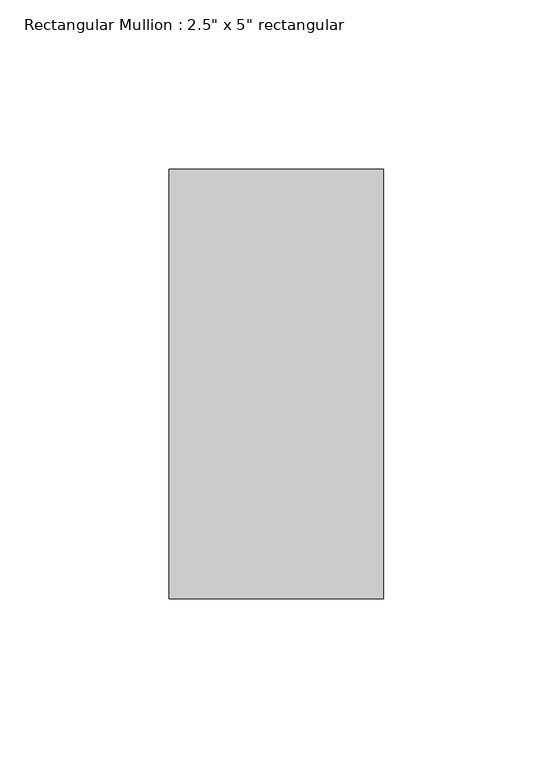
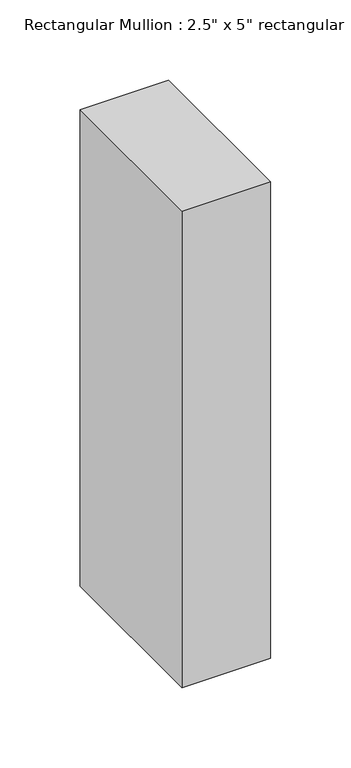
"""IFC4 building model written with IfcOpenShell, lengths in millimetres: member geometry."""

from ifc_helpers import new_model, si_unit, frame, origin, place, context, project, spatial, polyline, outline, extrude, source, transform, mapped, element, save


def member_af2f84b9(model_context):
    return source(origin(), model_context, "Body", "SweptSolid", [
        extrude(outline(polyline([(31.75, 63.5), (31.75, -63.5), (-31.75, -63.5), (-31.75, 63.5), (31.75, 63.5)])), frame((0.0, 0.0, -361.95), z_axis=(0.0, 0.0, 1.0), x_axis=(1.0, 0.0, 0.0)), (0.0, 0.0, 1.0), 361.95),
    ])


if __name__ == "__main__":
    model = new_model("IFC4")
    model_context = context("Model", 3, world=origin())
    ifc_project = project(units=[si_unit("LENGTHUNIT", "METRE", prefix="MILLI")], contexts=[model_context])
    site = spatial("IfcSite", under=ifc_project)
    building = spatial("IfcBuilding", under=site)
    placement = place(None, origin())
    member_shape = member_af2f84b9(model_context)
    element("IfcMember", 1, ObjectType="Rectangular Mullion : 2.5\" x 5\" rectangular", at=placement, inside=building, context=model_context, shape_type="MappedRepresentation", body=[
        mapped(member_shape, transform((0.0, 0.0, 0.0), x_axis=(1.0, 0.0, 0.0), y_axis=(0.0, 1.0, 0.0), z_axis=(0.0, 0.0, 1.0))),
    ])
    save(model, "model.ifc")

# Revit data of these elements
# Type "Rectangular Mullion : 2.5\" x 5\" rectangular"
#   built-in parameter 1007304 = 0.416667 (stored number, unit not read)
#   built-in parameter 1007301 = 0.104167 (stored number, unit not read)
#   built-in parameter 1007300 = 0.104167 (stored number, unit not read)
